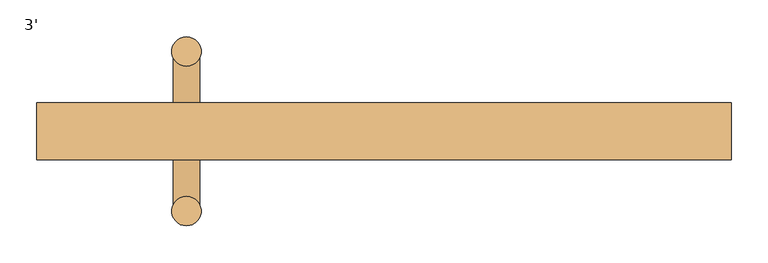
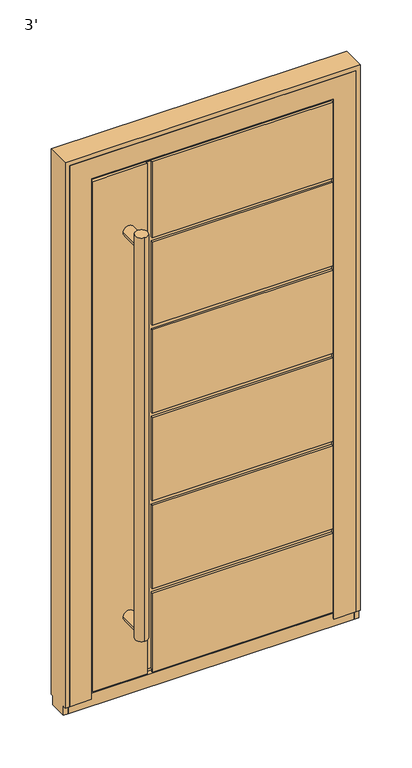
"""IFC4 building model written with IfcOpenShell, lengths in millimetres: door geometry, 3'."""

from ifc_helpers import new_model, si_unit, point, frame, frame_2d, origin, place, context, project, spatial, circle_curve, trimmed, segment, composite_curve, outline, extrude, faceted_brep, source, transform, mapped, element, save


def door_3_ad1505b7(model_context):
    return source(origin(), model_context, "Body", "SolidModel", [
        extrude(outline(composite_curve([segment(trimmed(circle_curve(frame_2d((-268.65, -90.8003001)), 20.0), [point((-268.65, -70.8003001))], [point((-268.65, -110.8003001))], False, "CARTESIAN"), True, "CONTINUOUS"), segment(trimmed(circle_curve(frame_2d((-268.65, -90.8003001)), 20.0), [point((-268.65, -110.8003001))], [point((-268.65, -70.8003001))], False, "CARTESIAN"), True, "CONTINUOUS")], self_intersect=False)), frame((0.0, 0.0, 210.0000003), z_axis=(0.0, 0.0, 1.0), x_axis=(1.0, 0.0, 0.0)), (0.0, 0.0, 1.0), 1363.8),
        extrude(outline(composite_curve([segment(trimmed(circle_curve(frame_2d((-268.65, 126.2003001)), 20.0), [point((-268.65, 146.2003001))], [point((-268.65, 106.2003001))], False, "CARTESIAN"), True, "CONTINUOUS"), segment(trimmed(circle_curve(frame_2d((-268.65, 126.2003001)), 20.0), [point((-268.65, 106.2003001))], [point((-268.65, 146.2003001))], False, "CARTESIAN"), True, "CONTINUOUS")], self_intersect=False)), frame((0.0, 0.0, 210.0000003), z_axis=(0.0, 0.0, 1.0), x_axis=(1.0, 0.0, 0.0)), (0.0, 0.0, 1.0), 1363.8),
        extrude(outline(composite_curve([segment(trimmed(circle_curve(frame_2d((241.9000003, -268.65)), 18.0), [point((241.9000003, -286.65))], [point((241.9000003, -250.65))], False, "CARTESIAN"), True, "CONTINUOUS"), segment(trimmed(circle_curve(frame_2d((241.9000003, -268.65)), 18.0), [point((241.9000003, -250.65))], [point((241.9000003, -286.65))], False, "CARTESIAN"), True, "CONTINUOUS")], self_intersect=False)), frame((0.0, -90.8, 0.0), z_axis=(0.0, 1.0, 0.0), x_axis=(0.0, 0.0, 1.0)), (0.0, 0.0, 1.0), 217.0),
        extrude(outline(composite_curve([segment(trimmed(circle_curve(frame_2d((1541.9000003, -268.65)), 18.0), [point((1541.9000003, -286.65))], [point((1541.9000003, -250.65))], False, "CARTESIAN"), True, "CONTINUOUS"), segment(trimmed(circle_curve(frame_2d((1541.9000003, -268.65)), 18.0), [point((1541.9000003, -250.65))], [point((1541.9000003, -286.65))], False, "CARTESIAN"), True, "CONTINUOUS")], self_intersect=False)), frame((0.0, -90.8, 0.0), z_axis=(0.0, 1.0, 0.0), x_axis=(0.0, 0.0, 1.0)), (0.0, 0.0, 1.0), 217.0),
        faceted_brep([(-193.65, -13.8, 306.466667), (-193.65, -13.8, 587.9333337), (383.65, -13.8, 587.9333337), (383.65, -13.8, 602.9333337), (-193.65, -13.8, 602.9333337), (-193.65, -13.8, 884.4000004), (383.65, -13.8, 884.4000004), (383.65, -13.8, 899.4000004), (-193.65, -13.8, 899.4000004), (-193.65, -13.8, 1180.866667), (383.65, -13.8, 1180.866667), (383.65, -13.8, 1195.866667), (-193.65, -13.8, 1195.866667), (-193.65, -13.8, 1477.3333337), (383.65, -13.8, 1477.3333337), (383.65, -13.8, 1492.3333337), (-193.65, -13.8, 1492.3333337), (-193.65, -13.8, 1748.8000003), (-208.65, -13.8, 1748.8000003), (-208.65, -13.8, 35.0), (-193.65, -13.8, 35.0), (-193.65, -13.8, 291.466667), (383.65, -13.8, 291.466667), (383.65, -13.8, 306.466667), (-193.65, -20.8, 306.466667), (-193.65, -20.8, 587.9333337), (383.65, -20.8, 587.9333337), (383.65, -11.7997698, 1748.8000003), (383.65, -20.8, 1748.8000003), (383.65, -20.8, 1492.3333337), (383.65, -20.8, 1477.3333337), (383.65, -20.8, 1195.866667), (383.65, -20.8, 1180.866667), (383.65, -20.8, 899.4000004), (383.65, -20.8, 884.4000004), (383.65, -20.8, 602.9333337), (383.65, -20.8, 306.466667), (383.65, -20.8, 291.466667), (383.65, -20.8, 24.0), (383.65, -18.8020472, 24.0), (383.65, -18.8020472, 35.0), (383.65, -11.7997698, 35.0), (-193.65, -20.8, 602.9333337), (-193.65, -20.8, 884.4000004), (-193.65, -20.8, 899.4000004), (-193.65, -20.8, 1180.866667), (-208.65, -20.8, 1748.8000003), (-208.65, -20.8, 24.0), (-208.65, -18.8020472, 24.0), (-208.65, -18.8020472, 35.0), (-193.65, -18.8020472, 35.0), (-383.65, -18.8020472, 35.0), (-383.65, -11.7997698, 35.0), (-193.65, -20.8, 291.466667), (-193.65, -18.8020472, 24.0), (-193.65, -20.8, 24.0), (-383.65, -18.8020472, 24.0), (-383.65, -20.8, 24.0), (-383.65, -20.8, 1748.8000003), (-193.65, -20.8, 1477.3333337), (-193.65, -20.8, 1195.866667), (-193.65, -20.8, 1748.8000003), (-193.65, -20.8, 1492.3333337), (408.65, 56.2, 10.0000003), (408.65, 53.2, 10.0000003), (-193.65, 53.2, 10.0000003), (-193.65, 56.2, 10.0000003), (-408.65, 53.2, 10.0000003), (-408.65, 56.2, 10.0000003), (-208.65, 56.2, 10.0000003), (-208.65, 53.2, 10.0000003), (408.65, 56.2, 291.466667), (408.65, 53.2, 291.466667), (408.65, 56.2, 306.466667), (408.65, 56.2, 587.9333337), (408.65, 53.2, 587.9333337), (408.65, 53.2, 306.466667), (408.65, 56.2, 899.4000004), (408.65, 56.2, 1180.866667), (408.65, 53.2, 1180.866667), (408.65, 53.2, 899.4000004), (408.65, 56.2, 602.9333337), (408.65, 56.2, 884.4000004), (408.65, 53.2, 884.4000004), (408.65, 53.2, 602.9333337), (408.65, 56.2, 1195.866667), (408.65, 56.2, 1477.3333337), (408.65, 53.2, 1477.3333337), (408.65, 53.2, 1195.866667), (408.65, 56.2, 1773.8000003), (408.65, 53.2, 1773.8000003), (408.65, 53.2, 1492.3333337), (408.65, 56.2, 1492.3333337), (393.15, 53.2, 291.466667), (393.15, 53.2, 25.5), (-193.65, 53.2, 25.5), (393.15, 53.2, 587.9333337), (393.15, 53.2, 306.466667), (393.15, 53.2, 1180.866667), (393.15, 53.2, 899.4000004), (393.15, 53.2, 884.4000004), (393.15, 53.2, 602.9333337), (393.15, 53.2, 1477.3333337), (393.15, 53.2, 1195.866667), (-193.65, 53.2, 1773.8000003), (-193.65, 53.2, 1758.3000003), (393.15, 53.2, 1758.3000003), (393.15, 53.2, 1492.3333337), (-393.15, 53.2, 25.5), (-393.15, 53.2, 1758.3000003), (-208.65, 53.2, 1758.3000003), (-208.65, 53.2, 1773.8000003), (-408.65, 53.2, 1773.8000003), (-208.65, 53.2, 25.5), (-193.65, 49.2, 291.466667), (-193.65, 56.2, 291.466667), (-193.65, 49.2, 25.5), (-193.65, 56.2, 306.466667), (-193.65, 56.2, 587.9333337), (-193.65, 56.2, 899.4000004), (-193.65, 56.2, 1180.866667), (-193.65, 56.2, 602.9333337), (-193.65, 56.2, 884.4000004), (-193.65, 56.2, 1195.866667), (-193.65, 56.2, 1477.3333337), (-193.65, 56.2, 1492.3333337), (-193.65, 56.2, 1773.8000003), (-408.65, 56.2, 1773.8000003), (-208.65, 56.2, 1773.8000003), (-208.65, 49.2, 1758.3000003), (-208.65, 49.2, 25.5), (-383.65, -11.7997698, 1748.8000003), (393.15, -11.7997698, 1758.3000003), (-393.15, -11.7997698, 1758.3000003), (-393.15, -11.7997698, 25.5), (393.15, -11.7997698, 25.5), (393.15, 49.2, 291.466667), (393.15, 49.2, 306.466667), (393.15, 49.2, 587.9333337), (393.15, 49.2, 602.9333337), (393.15, 49.2, 884.4000004), (393.15, 49.2, 899.4000004), (393.15, 49.2, 1180.866667), (393.15, 49.2, 1195.866667), (393.15, 49.2, 1477.3333337), (393.15, 49.2, 1492.3333337), (-193.65, 49.2, 1477.3333337), (-193.65, 49.2, 1195.866667), (-193.65, 49.2, 1180.866667), (-193.65, 49.2, 899.4000004), (-193.65, 49.2, 884.4000004), (-193.65, 49.2, 602.9333337), (-193.65, 49.2, 587.9333337), (-193.65, 49.2, 306.466667), (-193.65, 49.2, 1758.3000003), (-193.65, 49.2, 1492.3333337)], [[[0, 1, 2, 3, 4, 5, 6, 7, 8, 9, 10, 11, 12, 13, 14, 15, 16, 17, 18, 19, 20, 21, 22, 23]], [[1, 0, 24, 25]], [[1, 25, 26, 2]], [[27, 28, 29, 15, 14, 30, 31, 11, 10, 32, 33, 7, 6, 34, 35, 3, 2, 26, 36, 23, 22, 37, 38, 39, 40, 41]], [[42, 4, 3, 35]], [[5, 4, 42, 43]], [[5, 43, 34, 6]], [[44, 8, 7, 33]], [[9, 8, 44, 45]], [[19, 18, 46, 47, 48, 49]], [[41, 40, 50, 20, 19, 49, 51, 52]], [[53, 21, 20, 50, 54, 55]], [[21, 53, 37, 22]], [[24, 0, 23, 36]], [[40, 39, 54, 50]], [[56, 51, 49, 48]], [[39, 38, 55, 54]], [[57, 56, 48, 47]], [[33, 32, 45, 44]], [[35, 34, 43, 42]], [[36, 26, 25, 24]], [[55, 38, 37, 53]], [[58, 57, 47, 46]], [[31, 30, 59, 60]], [[28, 61, 62, 29]], [[63, 64, 65, 66]], [[67, 68, 69, 70]], [[64, 63, 71, 72]], [[73, 74, 75, 76]], [[77, 78, 79, 80]], [[81, 82, 83, 84]], [[85, 86, 87, 88]], [[89, 90, 91, 92]], [[65, 64, 72, 93, 94, 95]], [[76, 75, 96, 97]], [[80, 79, 98, 99]], [[84, 83, 100, 101]], [[88, 87, 102, 103]], [[90, 104, 105, 106, 107, 91]], [[108, 109, 110, 111, 112, 67, 70, 113]], [[114, 115, 66, 65, 95, 116]], [[63, 66, 115, 71]], [[74, 73, 117, 118]], [[78, 77, 119, 120]], [[82, 81, 121, 122]], [[86, 85, 123, 124]], [[89, 92, 125, 126]], [[68, 127, 128, 69]], [[68, 67, 112, 127]], [[129, 130, 113, 70, 69, 128, 111, 110]], [[58, 131, 52, 51, 56, 57]], [[132, 133, 134, 135], [131, 27, 41, 52]], [[106, 132, 135, 94, 93, 136, 137, 97, 96, 138, 139, 101, 100, 140, 141, 99, 98, 142, 143, 103, 102, 144, 145, 107]], [[94, 135, 134, 108, 113, 130, 116, 95]], [[133, 109, 108, 134]], [[146, 147, 143, 142, 148, 149, 141, 140, 150, 151, 139, 138, 152, 153, 137, 136, 114, 116, 130, 129, 154, 155, 145, 144]], [[149, 148, 120, 119]], [[149, 119, 77, 80, 99, 141]], [[122, 150, 140, 100, 83, 82]], [[151, 150, 122, 121]], [[151, 121, 81, 84, 101, 139]], [[118, 152, 138, 96, 75, 74]], [[153, 152, 118, 117]], [[153, 117, 73, 76, 97, 137]], [[115, 114, 136, 93, 72, 71]], [[9, 45, 32, 10]], [[60, 12, 11, 31]], [[13, 12, 60, 59]], [[13, 59, 30, 14]], [[62, 16, 15, 29]], [[16, 62, 61, 17]], [[124, 146, 144, 102, 87, 86]], [[125, 155, 154, 105, 104, 126]], [[120, 148, 142, 98, 79, 78]], [[147, 123, 85, 88, 103, 143]], [[147, 146, 124, 123]], [[155, 125, 92, 91, 107, 145]], [[90, 89, 126, 104]], [[127, 112, 111, 128]], [[132, 106, 105, 154, 129, 110, 109, 133]], [[27, 131, 58, 46, 18, 17, 61, 28]]]),
        faceted_brep([(-457.2, 56.2, 0.0), (-412.7, 56.2, 0.0), (-412.7, 47.2, 0.0), (-457.2, 47.1997571, 0.0), (-403.2, -16.2999958, 0.0), (-387.7, -16.2999958, 0.0), (-387.7, -20.8, 0.0), (-457.2, -20.8, 0.0), (-457.2, -11.8, 0.0), (-403.2, -11.8, 0.0), (457.2, -20.8, 0.0), (387.7, -20.8, 0.0), (387.7, -16.2999958, 0.0), (403.2, -16.2999958, 0.0), (403.2, -11.8, 0.0), (457.2, -11.8, 0.0), (412.7, 47.2, 0.0), (412.7, 56.2, 0.0), (457.2, 56.2, 0.0), (457.2, 47.1997571, 0.0), (-457.2, -20.8, 1828.8), (-457.2, 56.2, 1828.8), (-457.2, 47.1997571, -30.0), (-457.2, -11.8, -30.0), (457.2, 56.2, 1828.8), (412.7, 56.2, 1784.3), (-412.7, 56.2, 1784.3), (457.2, -20.8, 1828.8), (457.2, -11.8, -30.0), (457.2, 47.1997571, -30.0), (-387.7, -20.8, 1759.3), (387.7, -20.8, 1759.3), (-403.2, 47.2, 1774.8), (-403.2, -16.2999958, 1774.8), (-403.2, -11.8, 14.5), (-403.2, 47.2, 14.5), (403.2, 47.2, 1774.8), (403.2, -16.2999958, 1774.8), (403.2, 47.2, 14.5), (403.2, -11.8, 14.5), (-412.7, 47.2, 1784.3), (412.7, 47.2, 1784.3), (387.7, -16.2999958, 1759.3), (-387.7, -16.2999958, 1759.3)], [[[0, 1, 2, 3]], [[4, 5, 6, 7, 8, 9]], [[10, 11, 12, 13, 14, 15]], [[16, 17, 18, 19]], [[7, 20, 21, 0, 3, 22, 23, 8]], [[1, 0, 21, 24, 18, 17, 25, 26]], [[21, 20, 27, 24]], [[18, 24, 27, 10, 15, 28, 29, 19]], [[7, 6, 30, 31, 11, 10, 27, 20]], [[32, 33, 4, 9, 34, 35]], [[33, 32, 36, 37]], [[37, 36, 38, 39, 14, 13]], [[40, 2, 1, 26]], [[16, 19, 29, 22, 3, 2, 40, 41], [36, 32, 35, 38]], [[5, 4, 33, 37, 13, 12, 42, 43]], [[6, 5, 43, 30]], [[26, 25, 41, 40]], [[31, 30, 43, 42]], [[17, 16, 41, 25]], [[12, 11, 31, 42]], [[23, 28, 15, 14, 39, 34, 9, 8]], [[38, 35, 34, 39]], [[23, 22, 29, 28]]]),
        faceted_brep([(-457.2, 47.2, -30.0), (-457.2, -11.8, -30.0), (-472.2, -11.8, -30.0), (-472.2, 47.2, -30.0), (-457.2, 56.2, 1828.8), (-457.2, -20.8, 1828.8), (-457.2, -20.8, 0.0), (-457.2, -11.8, 0.0), (-457.2, 47.2, 0.0), (-457.2, 56.2, 0.0), (472.2, -11.8, 0.0), (457.2, -11.8, 0.0), (457.2, -11.8, -30.0), (472.2, -11.8, -30.0), (-472.2, -11.8, 0.0), (-472.2, -20.8, 1843.8), (-472.2, 56.2, 1843.8), (-472.2, 56.2, 0.0), (-472.2, 47.2, 0.0), (-472.2, -20.8, 0.0), (457.2, 47.2, 0.0), (472.2, 47.2, 0.0), (472.2, 47.2, -30.0), (457.2, 47.2, -30.0), (457.2, -20.8, 1828.8), (457.2, 56.2, 1828.8), (457.2, 56.2, 0.0), (457.2, -20.8, 0.0), (472.2, 56.2, 1843.8), (472.2, 56.2, 0.0), (472.2, -20.8, 0.0), (472.2, -20.8, 1843.8)], [[[0, 1, 2, 3]], [[4, 5, 6, 7, 1, 0, 8, 9]], [[10, 11, 12, 13]], [[7, 14, 2, 1]], [[15, 16, 17, 18, 3, 2, 14, 19]], [[20, 21, 22, 23]], [[18, 8, 0, 3]], [[24, 25, 26, 20, 23, 12, 11, 27]], [[25, 4, 9, 17, 16, 28, 29, 26]], [[21, 20, 26, 29]], [[8, 18, 17, 9]], [[22, 13, 12, 23]], [[11, 10, 30, 27]], [[14, 7, 6, 19]], [[5, 24, 27, 30, 31, 15, 19, 6]], [[28, 31, 30, 10, 13, 22, 21, 29]], [[5, 4, 25, 24]], [[16, 15, 31, 28]]]),
    ])


if __name__ == "__main__":
    model = new_model("IFC4")
    model_context = context("Model", 3, world=origin())
    ifc_project = project(units=[si_unit("LENGTHUNIT", "METRE", prefix="MILLI")], contexts=[model_context])
    site = spatial("IfcSite", under=ifc_project)
    building = spatial("IfcBuilding", under=site)
    placement = place(None, origin())
    door_3_shape = door_3_ad1505b7(model_context)
    element("IfcDoor", 1, ObjectType="3'", at=placement, inside=building, context=model_context, shape_type="MappedRepresentation", body=[
        mapped(door_3_shape, transform((0.0, 0.0, 0.0), x_axis=(1.0, 0.0, 0.0), y_axis=(0.0, 1.0, 0.0), z_axis=(0.0, 0.0, 1.0))),
    ])
    save(model, "model.ifc")

# Revit data of these elements
# Type "3'"
#   Type Mark = "9"
#   Water resistance = "up to Class E900, EN 12208:2001"
#   Uniclass2015Version = "v1.21"
#   Uniclass2015Reference = "Ss_25_30_20_30"
#   Uniclass2015Description = "Frame and door leaf system"
#   URL = "www.aluprof.com"
#   Type IFC Predefined Type = "USERDEFINED"
#   Right-hand / Left-hand door [instance default] = ""
#   Resistance to wind load = "up to Class C5/B5, EN 12210:2001"
#   Insert type = "ST"
#   Hardware [instance default] = ""
#   Product page = "https://aluprof.com/en/architects/offer/window-and-door-systems/panel-doors#visualisation"
#   Operation = "SinglePanelOutwardOpening"
#   Opening type = "Outward"
#   NBSReference = "25-50-20/125"
#   NBSDescription = "Frame and door leaf system"
#   Important = "The actual acceptable construction dimensions are dependent on the selection of profiles and hardware, glazing type, construction weight and the construction’s operating conditions. These should be determined by a suitably qualified person, and using ALUPROF’s calculation software"
#   IfcExportType = "USERDEFINED"
#   IfcExportAs = "IfcDoorType"
#   Handle type [instance default] = ""
#   Manufacturer = "ALUPROF SA"
#   Export Type to IFC As = "IfcDoorType"
#   Door sill type [instance default] = ""
#   Description = "External single-leaf panel door outward opening"
#   Model = "MB-86 ST Panel Door AD07"
#   Content of the recyclate in the material = "69.2%"
#   COBie.Type.WarrantyDurationParts = ""
#   COBie.Type.Name = ""
#   COBie.Type.Manufacturer = "ALUPROF SA"
#   COBie.Space.Name = ""
#   COBie.Floor.Name = ""
#   COBie.Facility.Name = ""
#   COBie.CreatedOn = ""
#   COBie.Component.WarrantyStartDate = ""
#   COBie.Component.Name = "MB-86 ST Panel Door AD07"
#   Burglar resistance = "RC2"
#   Air permeability = "up to Class 4, EN 12207:2001"
#   Width of the active leaf = 2' - 8.17717"
#   Placement in wall = 0' - 0.7874"
#   Thickness = 0' - 3.0315"
#   Height of the opening sash = 5' - 9.44094"
#   Handle Offset = 3' - 5.33858"
#   Rough Height = 6' - 2.40945"
#   Rough Width = 3' - 1.1811"
#   Height = 6' - 0"
#   Width = 3' - 0"
#   Construction depth = 0' - 3.0315"
#   Clear opening width = 2' - 3.94882"
#   Clear opening height = 5' - 8.47638"
#   Height of the array = 0' - 11.08136"
#   Schedule No. [instance default] = 1
#   Handrail [instance default] = yes
#   IsExternal = yes
#   Handle [instance default] = no
#   Door closer [instance default] = no
#   Function = 1
#   COBie.Type = yes
#   COBie = yes
#   Access control [instance default] = no
#   Panel = element 380416
#   Wall Closure = (empty or 0)
